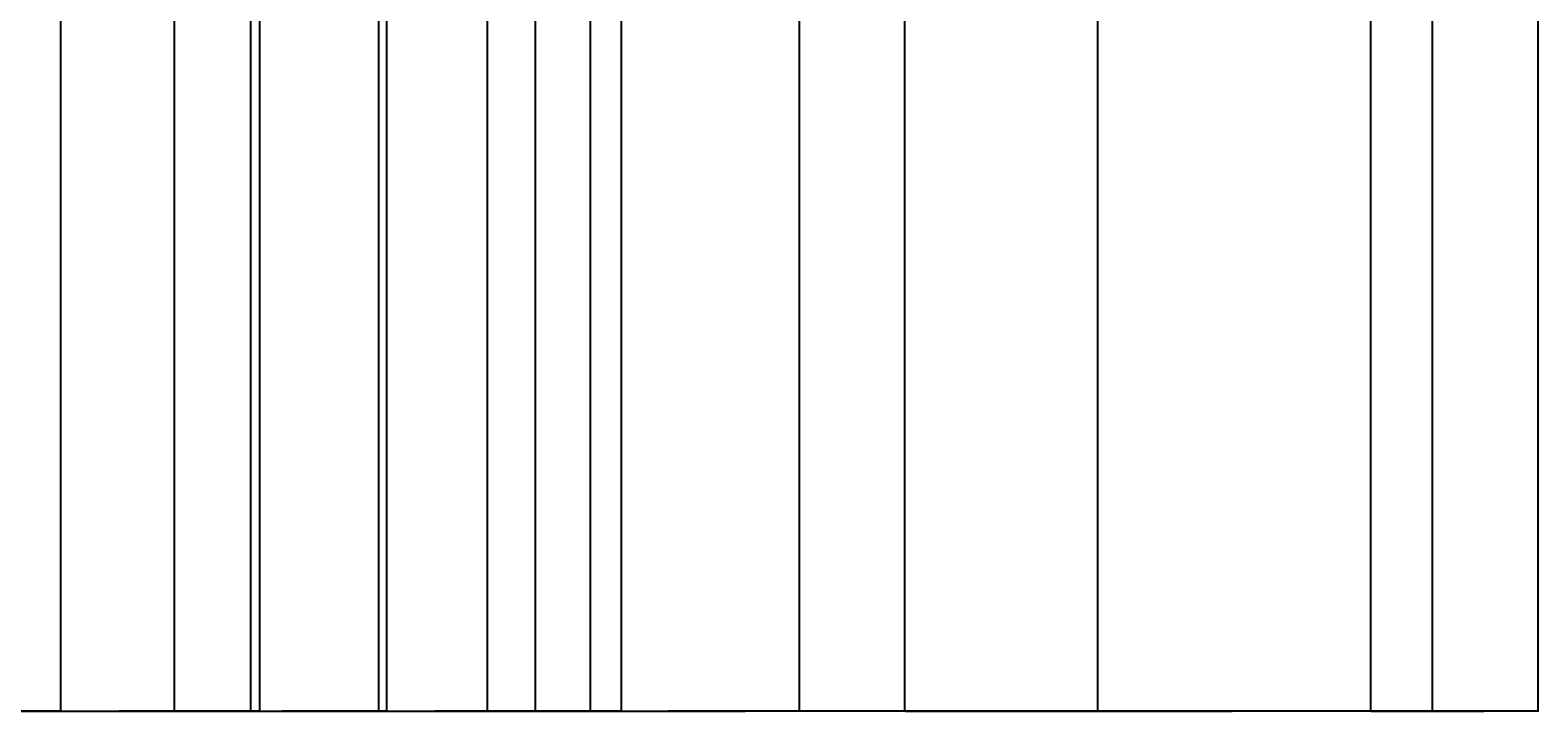
# Model space of a CAD drawing. Units: inches. Extents: x 484 to 1264, y 95 to 991.
# Tile 2 of 8: x 657 to 1000, y 95 to 250. Entities that reach past the tile are written whole.
import ezdxf

# ---------------------------------------------------------------- set-up
doc = ezdxf.new("R2010")
doc.units = ezdxf.units.IN
doc.header["$MEASUREMENT"] = 0
doc.layers.add('A-ANNO-DIMS', color=2, linetype='Continuous', lineweight=18)
doc.styles.get("Standard").update_dxf_attribs({"font": 'arial.ttf'})
doc.dimstyles.get("Standard").update_dxf_attribs({"dimtxt": 0.18, "dimasz": 0.18, "dimexe": 0.18, "dimexo": 0.0625, "dimgap": 0.09, "dimtad": 0, "dimtih": 1, "dimtoh": 1, "dimdec": 4, "dimzin": 0, "dimdsep": 46, "dimtxsty": 'Standard', "dimcen": 0.09, "dimadec": 0, "dimazin": 0, "dimtfac": 1, "dimtdec": 4, "dimtofl": 0, "dimtmove": 0, "dimatfit": 3, "dimfxl": 1, "dimtolj": 1, "dimtzin": 0, "dimarcsym": 0})

# ---------------------------------------------------------------- blocks, each defined once
blk = doc.blocks.new('*D16')
at = {"layer": 'A-ANNO-DIMS', "color": 0, "lineweight": -2, "transparency": 16777216}
for p, q in [((639.81, 408.32), (639.81, 94.79)), ((999.81, 318.32), (999.81, 94.79)), ((639.99, 94.97), (819.53, 94.97)), ((999.63, 94.97), (820.1, 94.97))]:
    blk.add_line(p, q, dxfattribs=at)
at = {"layer": 'A-ANNO-DIMS', "color": 0, "transparency": 16777216}
for points in [[(639.99, 95), (639.99, 94.94), (639.81, 94.97)], [(999.63, 95), (999.63, 94.94), (999.81, 94.97)]]:
    blk.add_solid(points, dxfattribs=at)
at = {"layer": 'Defpoints', "color": 0, "transparency": 16777216}
for p in [(639.81, 408.38), (999.81, 318.38), (999.81, 94.97)]:
    blk.add_point(p, dxfattribs=at)
at = {"layer": 'A-ANNO-DIMS', "color": 0, "transparency": 16777216, "insert": (819.81, 94.97), "char_height": 0.18, "attachment_point": 5}
blk.add_mtext('\\A1;360', dxfattribs=at)
blk = doc.blocks.new('*D23')
at = {"layer": 'A-ANNO-DIMS', "color": 0, "lineweight": -2, "transparency": 16777216}
for p, q in [((663.81, 906.32), (663.81, 94.79)), ((709.07, 889.06), (709.07, 94.79)), ((663.99, 94.97), (686.04, 94.97)), ((708.89, 94.97), (686.84, 94.97))]:
    blk.add_line(p, q, dxfattribs=at)
at = {"layer": 'A-ANNO-DIMS', "color": 0, "transparency": 16777216}
for points in [[(663.99, 95), (663.99, 94.94), (663.81, 94.97)], [(708.89, 95), (708.89, 94.94), (709.07, 94.97)]]:
    blk.add_solid(points, dxfattribs=at)
at = {"layer": 'Defpoints', "color": 0, "transparency": 16777216}
for p in [(663.81, 906.38), (709.07, 889.12), (709.07, 94.97)]:
    blk.add_point(p, dxfattribs=at)
at = {"layer": 'A-ANNO-DIMS', "color": 0, "transparency": 16777216, "insert": (686.44, 94.97), "char_height": 0.18, "attachment_point": 5}
blk.add_mtext('\\A1;45.25', dxfattribs=at)
blk = doc.blocks.new('*D24')
at = {"layer": 'A-ANNO-DIMS', "color": 0, "lineweight": -2, "transparency": 16777216}
for p, q in [((709.07, 889.06), (709.07, 94.79)), ((736.12, 889.06), (736.12, 94.79)), ((709.25, 94.97), (722.2, 94.97)), ((735.94, 94.97), (722.99, 94.97))]:
    blk.add_line(p, q, dxfattribs=at)
at = {"layer": 'A-ANNO-DIMS', "color": 0, "transparency": 16777216}
for points in [[(709.25, 95), (709.25, 94.94), (709.07, 94.97)], [(735.94, 95), (735.94, 94.94), (736.12, 94.97)]]:
    blk.add_solid(points, dxfattribs=at)
at = {"layer": 'Defpoints', "color": 0, "transparency": 16777216}
for p in [(709.07, 889.12), (736.12, 889.12), (736.12, 94.97)]:
    blk.add_point(p, dxfattribs=at)
at = {"layer": 'A-ANNO-DIMS', "color": 0, "transparency": 16777216, "insert": (722.59, 94.97), "char_height": 0.18, "attachment_point": 5}
blk.add_mtext('\\A1;27.05', dxfattribs=at)
blk = doc.blocks.new('*D25')
at = {"layer": 'A-ANNO-DIMS', "color": 0, "lineweight": -2, "transparency": 16777216}
for p, q in [((736.12, 889.06), (736.12, 94.79)), ((760.87, 889.06), (760.87, 94.79)), ((736.3, 94.97), (748.1, 94.97)), ((760.69, 94.97), (748.89, 94.97))]:
    blk.add_line(p, q, dxfattribs=at)
at = {"layer": 'A-ANNO-DIMS', "color": 0, "transparency": 16777216}
for points in [[(736.3, 95), (736.3, 94.94), (736.12, 94.97)], [(760.69, 95), (760.69, 94.94), (760.87, 94.97)]]:
    blk.add_solid(points, dxfattribs=at)
at = {"layer": 'Defpoints', "color": 0, "transparency": 16777216}
for p in [(736.12, 889.12), (760.87, 889.12), (760.87, 94.97)]:
    blk.add_point(p, dxfattribs=at)
at = {"layer": 'A-ANNO-DIMS', "color": 0, "transparency": 16777216, "insert": (748.49, 94.97), "char_height": 0.18, "attachment_point": 5}
blk.add_mtext('\\A1;24.75', dxfattribs=at)
blk = doc.blocks.new('*D26')
at = {"layer": 'A-ANNO-DIMS', "color": 0, "lineweight": -2, "transparency": 16777216}
for p, q in [((689.66, 819.99), (689.66, 94.79)), ((663.81, 810.32), (663.81, 94.79)), ((663.99, 94.97), (676.27, 94.97)), ((689.48, 94.97), (677.2, 94.97))]:
    blk.add_line(p, q, dxfattribs=at)
at = {"layer": 'A-ANNO-DIMS', "color": 0, "transparency": 16777216}
for points in [[(663.99, 95), (663.99, 94.94), (663.81, 94.97)], [(689.48, 95), (689.48, 94.94), (689.66, 94.97)]]:
    blk.add_solid(points, dxfattribs=at)
at = {"layer": 'Defpoints', "color": 0, "transparency": 16777216}
for p in [(689.66, 820.06), (663.81, 810.38), (689.66, 94.97)]:
    blk.add_point(p, dxfattribs=at)
at = {"layer": 'A-ANNO-DIMS', "color": 0, "transparency": 16777216, "insert": (676.74, 94.97), "char_height": 0.18, "attachment_point": 5}
blk.add_mtext('\\A1;25.846', dxfattribs=at)
blk = doc.blocks.new('*D27')
at = {"layer": 'A-ANNO-DIMS', "color": 0, "lineweight": -2, "transparency": 16777216}
for p, q in [((689.66, 819.99), (689.66, 94.79)), ((737.98, 819.99), (737.98, 94.79)), ((689.84, 94.97), (713.42, 94.97)), ((737.8, 94.97), (714.22, 94.97))]:
    blk.add_line(p, q, dxfattribs=at)
at = {"layer": 'A-ANNO-DIMS', "color": 0, "transparency": 16777216}
for points in [[(689.84, 95), (689.84, 94.94), (689.66, 94.97)], [(737.8, 95), (737.8, 94.94), (737.98, 94.97)]]:
    blk.add_solid(points, dxfattribs=at)
at = {"layer": 'Defpoints', "color": 0, "transparency": 16777216}
for p in [(689.66, 820.06), (737.98, 820.06), (737.98, 94.97)]:
    blk.add_point(p, dxfattribs=at)
at = {"layer": 'A-ANNO-DIMS', "color": 0, "transparency": 16777216, "insert": (713.82, 94.97), "char_height": 0.18, "attachment_point": 5}
blk.add_mtext('\\A1;48.32', dxfattribs=at)
blk = doc.blocks.new('*D28')
at = {"layer": 'A-ANNO-DIMS', "color": 0, "lineweight": -2, "transparency": 16777216}
for p, q in [((737.98, 819.99), (737.98, 94.79)), ((784.3, 819.99), (784.3, 94.79)), ((738.16, 94.97), (760.67, 94.97)), ((784.12, 94.97), (761.61, 94.97))]:
    blk.add_line(p, q, dxfattribs=at)
at = {"layer": 'A-ANNO-DIMS', "color": 0, "transparency": 16777216}
for points in [[(738.16, 95), (738.16, 94.94), (737.98, 94.97)], [(784.12, 95), (784.12, 94.94), (784.3, 94.97)]]:
    blk.add_solid(points, dxfattribs=at)
at = {"layer": 'Defpoints', "color": 0, "transparency": 16777216}
for p in [(737.98, 820.06), (784.3, 820.06), (784.3, 94.97)]:
    blk.add_point(p, dxfattribs=at)
at = {"layer": 'A-ANNO-DIMS', "color": 0, "transparency": 16777216, "insert": (761.14, 94.97), "char_height": 0.18, "attachment_point": 5}
blk.add_mtext('\\A1;46.325', dxfattribs=at)
blk = doc.blocks.new('*D29')
at = {"layer": 'A-ANNO-DIMS', "color": 0, "lineweight": -2, "transparency": 16777216}
for p, q in [((831.81, 906.32), (831.81, 94.79)), ((784.3, 819.99), (784.3, 94.79)), ((784.48, 94.97), (807.68, 94.97)), ((831.63, 94.97), (808.44, 94.97))]:
    blk.add_line(p, q, dxfattribs=at)
at = {"layer": 'A-ANNO-DIMS', "color": 0, "transparency": 16777216}
for points in [[(784.48, 95), (784.48, 94.94), (784.3, 94.97)], [(831.63, 95), (831.63, 94.94), (831.81, 94.97)]]:
    blk.add_solid(points, dxfattribs=at)
at = {"layer": 'Defpoints', "color": 0, "transparency": 16777216}
for p in [(831.81, 906.38), (784.3, 820.06), (831.81, 94.97)]:
    blk.add_point(p, dxfattribs=at)
at = {"layer": 'A-ANNO-DIMS', "color": 0, "transparency": 16777216, "insert": (808.06, 94.97), "char_height": 0.18, "attachment_point": 5}
blk.add_mtext('\\A1;47.51', dxfattribs=at)
blk = doc.blocks.new('*D33')
at = {"layer": 'A-ANNO-DIMS', "color": 0, "lineweight": -2, "transparency": 16777216}
for p, q in [((639.81, 930.32), (639.81, 94.79)), ((663.81, 810.32), (663.81, 94.79)), ((639.99, 94.97), (651.59, 94.97)), ((663.63, 94.97), (652.03, 94.97))]:
    blk.add_line(p, q, dxfattribs=at)
at = {"layer": 'A-ANNO-DIMS', "color": 0, "transparency": 16777216}
for points in [[(639.99, 95), (639.99, 94.94), (639.81, 94.97)], [(663.63, 95), (663.63, 94.94), (663.81, 94.97)]]:
    blk.add_solid(points, dxfattribs=at)
at = {"layer": 'Defpoints', "color": 0, "transparency": 16777216}
for p in [(639.81, 930.38), (663.81, 810.38), (663.81, 94.97)]:
    blk.add_point(p, dxfattribs=at)
at = {"layer": 'A-ANNO-DIMS', "color": 0, "transparency": 16777216, "insert": (651.81, 94.97), "char_height": 0.18, "attachment_point": 5}
blk.add_mtext('\\A1;24', dxfattribs=at)
blk = doc.blocks.new('*D36')
at = {"layer": 'A-ANNO-DIMS', "color": 0, "lineweight": -2, "transparency": 16777216}
for p, q in [((707.04, 581.21), (707.04, 94.79)), ((663.81, 501.32), (663.81, 94.79)), ((663.99, 94.97), (685.03, 94.97)), ((706.86, 94.97), (685.82, 94.97))]:
    blk.add_line(p, q, dxfattribs=at)
at = {"layer": 'A-ANNO-DIMS', "color": 0, "transparency": 16777216}
for points in [[(663.99, 95), (663.99, 94.94), (663.81, 94.97)], [(706.86, 95), (706.86, 94.94), (707.04, 94.97)]]:
    blk.add_solid(points, dxfattribs=at)
at = {"layer": 'Defpoints', "color": 0, "transparency": 16777216}
for p in [(707.04, 581.28), (663.81, 501.38), (707.04, 94.97)]:
    blk.add_point(p, dxfattribs=at)
at = {"layer": 'A-ANNO-DIMS', "color": 0, "transparency": 16777216, "insert": (685.43, 94.97), "char_height": 0.18, "attachment_point": 5}
blk.add_mtext('\\A1;43.22', dxfattribs=at)
blk = doc.blocks.new('*D37')
at = {"layer": 'A-ANNO-DIMS', "color": 0, "lineweight": -2, "transparency": 16777216}
for p, q in [((707.04, 581.21), (707.04, 94.79)), ((791.36, 581.21), (791.36, 94.79)), ((707.22, 94.97), (748.81, 94.97)), ((791.18, 94.97), (749.59, 94.97))]:
    blk.add_line(p, q, dxfattribs=at)
at = {"layer": 'A-ANNO-DIMS', "color": 0, "transparency": 16777216}
for points in [[(707.22, 95), (707.22, 94.94), (707.04, 94.97)], [(791.18, 95), (791.18, 94.94), (791.36, 94.97)]]:
    blk.add_solid(points, dxfattribs=at)
at = {"layer": 'Defpoints', "color": 0, "transparency": 16777216}
for p in [(707.04, 581.28), (791.36, 581.28), (791.36, 94.97)]:
    blk.add_point(p, dxfattribs=at)
at = {"layer": 'A-ANNO-DIMS', "color": 0, "transparency": 16777216, "insert": (749.2, 94.97), "char_height": 0.18, "attachment_point": 5}
blk.add_mtext('\\A1;84.32', dxfattribs=at)
blk = doc.blocks.new('*D40')
at = {"layer": 'A-ANNO-DIMS', "color": 0, "lineweight": -2, "transparency": 16777216}
for p, q in [((899.68, 562.19), (899.68, 94.79)), ((961.76, 562.19), (961.76, 94.79)), ((899.86, 94.97), (930.33, 94.97)), ((961.58, 94.97), (931.12, 94.97))]:
    blk.add_line(p, q, dxfattribs=at)
at = {"layer": 'A-ANNO-DIMS', "color": 0, "transparency": 16777216}
for points in [[(899.86, 95), (899.86, 94.94), (899.68, 94.97)], [(961.58, 95), (961.58, 94.94), (961.76, 94.97)]]:
    blk.add_solid(points, dxfattribs=at)
at = {"layer": 'Defpoints', "color": 0, "transparency": 16777216}
for p in [(899.68, 562.26), (961.76, 562.26), (961.76, 94.97)]:
    blk.add_point(p, dxfattribs=at)
at = {"layer": 'A-ANNO-DIMS', "color": 0, "transparency": 16777216, "insert": (930.72, 94.97), "char_height": 0.18, "attachment_point": 5}
blk.add_mtext('\\A1;62.08', dxfattribs=at)
blk = doc.blocks.new('*D41')
at = {"layer": 'A-ANNO-DIMS', "color": 0, "lineweight": -2, "transparency": 16777216}
for p, q in [((961.76, 562.19), (961.76, 94.79)), ((999.81, 537.32), (999.81, 94.79)), ((961.94, 94.97), (980.39, 94.97)), ((999.63, 94.97), (981.18, 94.97))]:
    blk.add_line(p, q, dxfattribs=at)
at = {"layer": 'A-ANNO-DIMS', "color": 0, "transparency": 16777216}
for points in [[(961.94, 95), (961.94, 94.94), (961.76, 94.97)], [(999.63, 95), (999.63, 94.94), (999.81, 94.97)]]:
    blk.add_solid(points, dxfattribs=at)
at = {"layer": 'Defpoints', "color": 0, "transparency": 16777216}
for p in [(961.76, 562.26), (999.81, 537.38), (999.81, 94.97)]:
    blk.add_point(p, dxfattribs=at)
at = {"layer": 'A-ANNO-DIMS', "color": 0, "transparency": 16777216, "insert": (980.79, 94.97), "char_height": 0.18, "attachment_point": 5}
blk.add_mtext('\\A1;38.05', dxfattribs=at)
blk = doc.blocks.new('*D49')
at = {"layer": 'A-ANNO-DIMS', "color": 0, "lineweight": -2, "transparency": 16777216}
for p, q in [((855.81, 318.32), (855.81, 94.79)), ((975.81, 318.32), (975.81, 94.79)), ((855.99, 94.97), (915.53, 94.97)), ((975.63, 94.97), (916.09, 94.97))]:
    blk.add_line(p, q, dxfattribs=at)
at = {"layer": 'A-ANNO-DIMS', "color": 0, "transparency": 16777216}
for points in [[(855.99, 95), (855.99, 94.94), (855.81, 94.97)], [(975.63, 95), (975.63, 94.94), (975.81, 94.97)]]:
    blk.add_solid(points, dxfattribs=at)
at = {"layer": 'Defpoints', "color": 0, "transparency": 16777216}
for p in [(855.81, 318.38), (975.81, 318.38), (975.81, 94.97)]:
    blk.add_point(p, dxfattribs=at)
at = {"layer": 'A-ANNO-DIMS', "color": 0, "transparency": 16777216, "insert": (915.81, 94.97), "char_height": 0.18, "attachment_point": 5}
blk.add_mtext('\\A1;120', dxfattribs=at)
blk = doc.blocks.new('*D53')
at = {"layer": 'A-ANNO-DIMS', "color": 0, "lineweight": -2, "transparency": 16777216}
for p, q in [((771.81, 330.32), (771.81, 94.79)), ((831.81, 330.32), (831.81, 94.79)), ((771.99, 94.97), (801.6, 94.97)), ((831.63, 94.97), (802.03, 94.97))]:
    blk.add_line(p, q, dxfattribs=at)
at = {"layer": 'A-ANNO-DIMS', "color": 0, "transparency": 16777216}
for points in [[(771.99, 95), (771.99, 94.94), (771.81, 94.97)], [(831.63, 95), (831.63, 94.94), (831.81, 94.97)]]:
    blk.add_solid(points, dxfattribs=at)
at = {"layer": 'Defpoints', "color": 0, "transparency": 16777216}
for p in [(771.81, 330.38), (831.81, 330.38), (831.81, 94.97)]:
    blk.add_point(p, dxfattribs=at)
at = {"layer": 'A-ANNO-DIMS', "color": 0, "transparency": 16777216, "insert": (801.81, 94.97), "char_height": 0.18, "attachment_point": 5}
blk.add_mtext('\\A1;60', dxfattribs=at)
blk = doc.blocks.new('*D55')
at = {"layer": 'A-ANNO-DIMS', "color": 0, "lineweight": -2, "transparency": 16777216}
for p, q in [((975.81, 318.32), (975.81, 94.79)), ((999.81, 318.32), (999.81, 94.79)), ((975.99, 94.97), (987.59, 94.97)), ((999.63, 94.97), (988.03, 94.97))]:
    blk.add_line(p, q, dxfattribs=at)
at = {"layer": 'A-ANNO-DIMS', "color": 0, "transparency": 16777216}
for points in [[(975.99, 95), (975.99, 94.94), (975.81, 94.97)], [(999.63, 95), (999.63, 94.94), (999.81, 94.97)]]:
    blk.add_solid(points, dxfattribs=at)
at = {"layer": 'Defpoints', "color": 0, "transparency": 16777216}
for p in [(975.81, 318.38), (999.81, 318.38), (999.81, 94.97)]:
    blk.add_point(p, dxfattribs=at)
at = {"layer": 'A-ANNO-DIMS', "color": 0, "transparency": 16777216, "insert": (987.81, 94.97), "char_height": 0.18, "attachment_point": 5}
blk.add_mtext('\\A1;24', dxfattribs=at)

msp = doc.modelspace()

# ---------------------------------------------------------------- dimensions: what is measured, and where the dimension line sits
at = {"layer": 'A-ANNO-DIMS'}
for base, p1, p2, override, picture, middle in [((663.8147, 94.9714), (639.8147, 930.3846), (663.8147, 810.3846), {"dimdec": 0, "dimlfac": 1, "dimrnd": 0, "dimzin": 0, "dimdsep": 46, "dimlunit": 2}, '*D33', (651.8147, 94.9714)), ((709.0683, 94.9714), (663.8147, 906.3846), (709.0683, 889.1187), {"dimdec": 2, "dimlfac": 1, "dimrnd": 0, "dimzin": 0, "dimdsep": 46, "dimlunit": 2}, '*D23', (686.4415, 94.9714)), ((831.8147, 94.9714), (784.3024, 820.0562), (831.8147, 906.3846), {"dimdec": 2, "dimlfac": 1, "dimrnd": 0, "dimzin": 0, "dimdsep": 46, "dimlunit": 2}, '*D29', (808.0586, 94.9714)), ((736.12, 94.9714), (709.0683, 889.1187), (736.12, 889.1187), {"dimdec": 2, "dimlfac": 1, "dimrnd": 0, "dimzin": 0, "dimdsep": 46, "dimlunit": 2}, '*D24', (722.5941, 94.9714)), ((760.8695, 94.9714), (736.12, 889.1187), (760.8695, 889.1187), {"dimdec": 2, "dimlfac": 1, "dimrnd": 0, "dimzin": 0, "dimdsep": 46, "dimlunit": 2}, '*D25', (748.4947, 94.9714)), ((689.6604, 94.9714), (663.8147, 810.3846), (689.6604, 820.0562), {"dimdec": 3, "dimlfac": 1, "dimrnd": 0, "dimzin": 0, "dimdsep": 46, "dimlunit": 2}, '*D26', (676.7376, 94.9714)), ((737.9777, 94.9714), (689.6604, 820.0562), (737.9777, 820.0562), {"dimdec": 2, "dimlfac": 1, "dimrnd": 0, "dimzin": 0, "dimdsep": 46, "dimlunit": 2}, '*D27', (713.8191, 94.9714)), ((784.3024, 94.9714), (737.9777, 820.0562), (784.3024, 820.0562), {"dimdec": 3, "dimlfac": 1, "dimrnd": 0, "dimzin": 0, "dimdsep": 46, "dimlunit": 2}, '*D28', (761.1401, 94.9714)), ((707.038, 94.9714), (663.8147, 501.3846), (707.038, 581.2764), {"dimdec": 2, "dimlfac": 1, "dimrnd": 0, "dimzin": 0, "dimdsep": 46, "dimlunit": 2}, '*D36', (685.4263, 94.9714)), ((791.3605, 94.9714), (707.038, 581.2764), (791.3605, 581.2764), {"dimdec": 2, "dimlfac": 1, "dimrnd": 0, "dimzin": 0, "dimdsep": 46, "dimlunit": 2}, '*D37', (749.1992, 94.9714)), ((961.7639, 94.9714), (899.6817, 562.256), (961.7639, 562.256), {"dimdec": 2, "dimlfac": 1, "dimrnd": 0, "dimzin": 0, "dimdsep": 46, "dimlunit": 2}, '*D40', (930.7228, 94.9714)), ((999.8147, 94.9714), (961.7639, 562.256), (999.8147, 537.3846), {"dimdec": 2, "dimlfac": 1, "dimrnd": 0, "dimzin": 0, "dimdsep": 46, "dimlunit": 2}, '*D41', (980.7893, 94.9714)), ((999.8147, 94.9714), (639.8147, 408.3846), (999.8147, 318.3846), {"dimdec": 0, "dimlfac": 1, "dimrnd": 0, "dimzin": 0, "dimdsep": 46, "dimlunit": 2}, '*D16', (819.8147, 94.9714)), ((831.8147, 94.9714), (771.8147, 330.3846), (831.8147, 330.3846), {"dimdec": 0, "dimlfac": 1, "dimrnd": 0, "dimzin": 0, "dimdsep": 46, "dimlunit": 2}, '*D53', (801.8147, 94.9714)), ((975.8147, 94.9714), (855.8147, 318.3846), (975.8147, 318.3846), {"dimdec": 0, "dimlfac": 1, "dimrnd": 0, "dimzin": 0, "dimdsep": 46, "dimlunit": 2}, '*D49', (915.8147, 94.9714)), ((999.8147, 94.9714), (975.8147, 318.3846), (999.8147, 318.3846), {"dimdec": 0, "dimlfac": 1, "dimrnd": 0, "dimzin": 0, "dimdsep": 46, "dimlunit": 2}, '*D55', (987.8147, 94.9714))]:
    dim = msp.add_linear_dim(base=base, p1=p1, p2=p2, dimstyle='Standard', override=override, dxfattribs=at)
    dim.commit()
    dim.dimension.update_dxf_attribs({"geometry": picture, "text_midpoint": middle})

doc.saveas('drawing.dxf')
